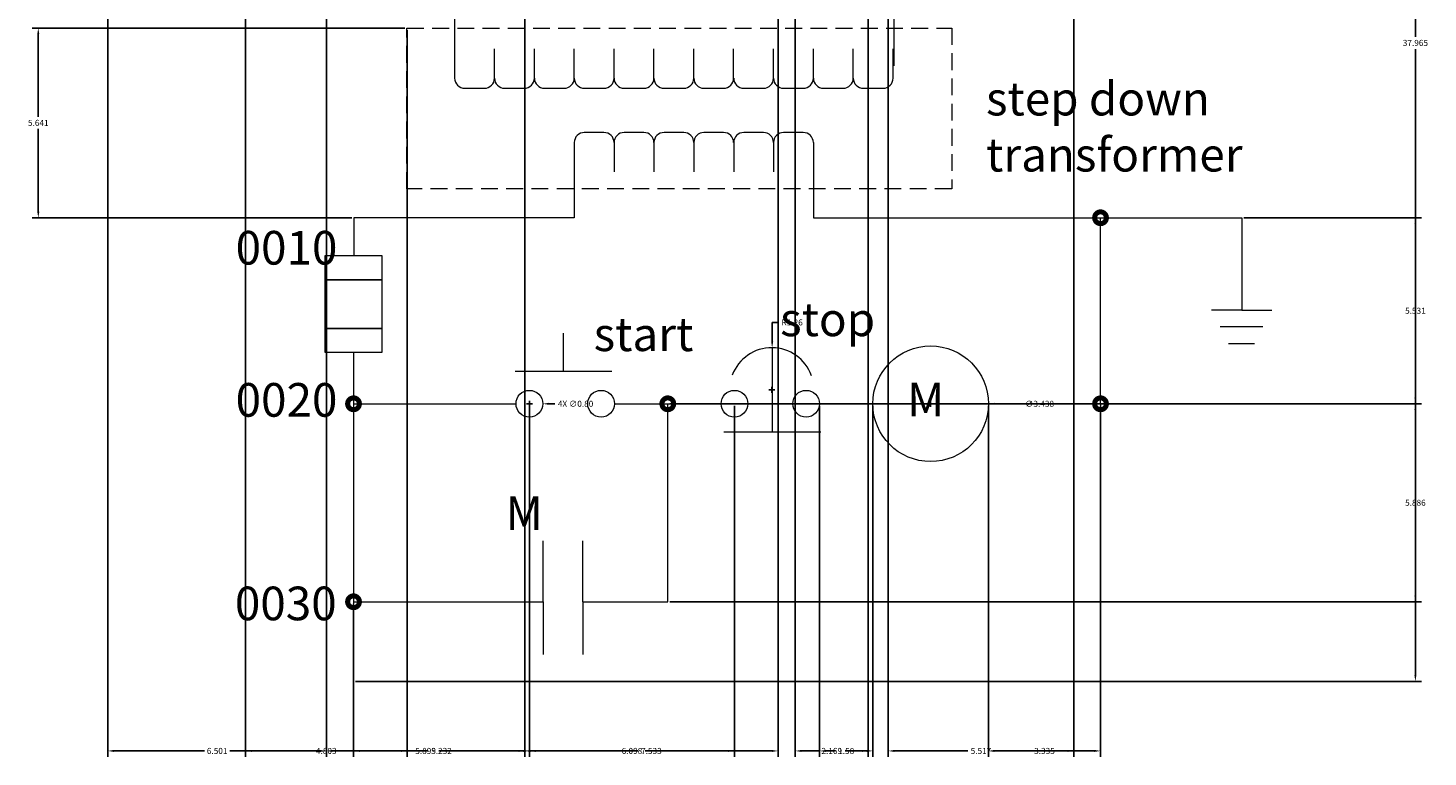
# Model space of a CAD drawing. Units: millimetres. Extents: x 39.4 to 81, y 9.5 to 52.5.
# Tile 1 of 2: x 39.4 to 81, y 9.5 to 31.2. Entities that reach past the tile are written whole.
import ezdxf

# ---------------------------------------------------------------- set-up
doc = ezdxf.new("R2010")
doc.units = ezdxf.units.MM
doc.header["$MEASUREMENT"] = 0
doc.linetypes.add('HIDDENX2', pattern=[0.75, 0.5, -0.25])
for name, color, linetype, lineweight in [('A-ANNO-DIMS', 2, 'Continuous', 18), ('E-ANNO-TEXT', 7, 'Continuous', 13), ('E-CTRL-DEVC', 7, 'Continuous', 18), ('E-CTRL-WIRE', 7, 'Continuous', 13), ('E-DIAG-CONN', 7, 'Continuous', 18), ('E-DIAG-PROT', 7, 'Continuous', 18), ('E-EQPM-BNDY', 8, 'HIDDENX2', 13), ('E-POWR-GRND', 7, 'Continuous', 18), ('E-POWR-WIRE', 7, 'Continuous', 18), ('E-POWR-XFMR', 7, 'Continuous', 18)]:
    doc.layers.add(name, color=color, linetype=linetype, lineweight=lineweight)
doc.styles.get("Standard").update_dxf_attribs({"font": 'arial.ttf'})
doc.dimstyles.get("Standard").update_dxf_attribs({"dimtxt": 0.18, "dimasz": 0.18, "dimexe": 0.18, "dimexo": 0.0625, "dimgap": 0.09, "dimtad": 0, "dimtih": 1, "dimtoh": 1, "dimdec": 4, "dimzin": 0, "dimdsep": 46, "dimtxsty": 'Standard', "dimcen": 0.09, "dimadec": 0, "dimazin": 0, "dimtfac": 1, "dimtdec": 4, "dimtofl": 0, "dimtmove": 0, "dimatfit": 3, "dimfxl": 1, "dimtolj": 1, "dimtzin": 0, "dimarcsym": 0})

# ---------------------------------------------------------------- blocks, each defined once
blk = doc.blocks.new('WIRE-JUNCTION')
at = {"const_width": 0.15}
blk.add_lwpolyline([(0, 0.175, 1), (0.35, 0.175, 1)], format="xyb", close=True, dxfattribs=at)
blk = doc.blocks.new('*D9')
at = {"layer": 'A-ANNO-DIMS', "color": 0, "lineweight": -2, "transparency": 16777216}
for p, q in [((50.604, 31.159), (39.52, 31.159)), ((39.7, 30.979), (39.7, 28.521)), ((39.7, 25.698), (39.7, 28.157)), ((49.021, 25.518), (39.52, 25.518))]:
    blk.add_line(p, q, dxfattribs=at)
at = {"layer": 'A-ANNO-DIMS', "color": 0, "transparency": 16777216}
for points in [[(39.67, 30.979), (39.73, 30.979), (39.7, 31.159)], [(39.67, 25.698), (39.73, 25.698), (39.7, 25.518)]]:
    blk.add_solid(points, dxfattribs=at)
at = {"layer": 'Defpoints', "color": 0, "transparency": 16777216}
for p in [(50.667, 31.159), (39.7, 25.518), (49.084, 25.518)]:
    blk.add_point(p, dxfattribs=at)
at = {"layer": 'A-ANNO-DIMS', "color": 0, "transparency": 16777216, "insert": (39.7, 28.339), "char_height": 0.18, "attachment_point": 5}
blk.add_mtext('\\A1;5.641', dxfattribs=at)
blk = doc.blocks.new('*D10')
at = {"layer": 'A-ANNO-DIMS', "color": 0, "lineweight": -2, "transparency": 16777216}
for p, q in [((75.556, 25.518), (80.841, 25.518)), ((80.661, 25.338), (80.661, 22.935)), ((80.661, 20.167), (80.661, 22.571)), ((71.358, 19.987), (80.841, 19.987))]:
    blk.add_line(p, q, dxfattribs=at)
at = {"layer": 'A-ANNO-DIMS', "color": 0, "transparency": 16777216}
for points in [[(80.631, 25.338), (80.691, 25.338), (80.661, 25.518)], [(80.631, 20.167), (80.691, 20.167), (80.661, 19.987)]]:
    blk.add_solid(points, dxfattribs=at)
at = {"layer": 'Defpoints', "color": 0, "transparency": 16777216}
for p in [(75.494, 25.518), (71.295, 19.987), (80.661, 19.987)]:
    blk.add_point(p, dxfattribs=at)
at = {"layer": 'A-ANNO-DIMS', "color": 0, "transparency": 16777216, "insert": (80.661, 22.753), "char_height": 0.18, "attachment_point": 5}
blk.add_mtext('\\A1;5.531', dxfattribs=at)
blk = doc.blocks.new('*D11')
at = {"layer": 'A-ANNO-DIMS', "color": 0, "lineweight": -2, "transparency": 16777216}
for p, q in [((58.486, 19.987), (80.841, 19.987)), ((80.661, 19.807), (80.661, 17.226)), ((80.661, 14.282), (80.661, 16.863)), ((58.486, 14.102), (80.841, 14.102))]:
    blk.add_line(p, q, dxfattribs=at)
at = {"layer": 'A-ANNO-DIMS', "color": 0, "transparency": 16777216}
for points in [[(80.631, 19.807), (80.691, 19.807), (80.661, 19.987)], [(80.631, 14.282), (80.691, 14.282), (80.661, 14.102)]]:
    blk.add_solid(points, dxfattribs=at)
at = {"layer": 'Defpoints', "color": 0, "transparency": 16777216}
for p in [(58.424, 19.987), (58.424, 14.102), (80.661, 14.102)]:
    blk.add_point(p, dxfattribs=at)
at = {"layer": 'A-ANNO-DIMS', "color": 0, "transparency": 16777216, "insert": (80.661, 17.045), "char_height": 0.18, "attachment_point": 5}
blk.add_mtext('\\A1;5.886', dxfattribs=at)
blk = doc.blocks.new('*D12')
at = {"layer": 'A-ANNO-DIMS', "color": 0, "lineweight": -2, "transparency": 16777216}
for p, q in [((41.769, 37.833), (41.769, 9.486)), ((48.27, 37.833), (48.27, 9.486)), ((41.949, 9.666), (44.643, 9.666)), ((48.09, 9.666), (45.396, 9.666))]:
    blk.add_line(p, q, dxfattribs=at)
at = {"layer": 'A-ANNO-DIMS', "color": 0, "transparency": 16777216}
for points in [[(41.949, 9.696), (41.949, 9.636), (41.769, 9.666)], [(48.09, 9.696), (48.09, 9.636), (48.27, 9.666)]]:
    blk.add_solid(points, dxfattribs=at)
at = {"layer": 'Defpoints', "color": 0, "transparency": 16777216}
for p in [(41.769, 37.896), (48.27, 37.896), (48.27, 9.666)]:
    blk.add_point(p, dxfattribs=at)
at = {"layer": 'A-ANNO-DIMS', "color": 0, "transparency": 16777216, "insert": (45.02, 9.666), "char_height": 0.18, "attachment_point": 5}
blk.add_mtext('\\A1;6.501', dxfattribs=at)
blk = doc.blocks.new('*D13')
at = {"layer": 'A-ANNO-DIMS', "color": 0, "lineweight": -2, "transparency": 16777216}
for p, q in [((48.27, 37.833), (48.27, 9.486)), ((54.169, 37.833), (54.169, 9.486)), ((48.45, 9.666), (50.826, 9.666)), ((53.989, 9.666), (51.614, 9.666))]:
    blk.add_line(p, q, dxfattribs=at)
at = {"layer": 'A-ANNO-DIMS', "color": 0, "transparency": 16777216}
for points in [[(48.45, 9.696), (48.45, 9.636), (48.27, 9.666)], [(53.989, 9.696), (53.989, 9.636), (54.169, 9.666)]]:
    blk.add_solid(points, dxfattribs=at)
at = {"layer": 'Defpoints', "color": 0, "transparency": 16777216}
for p in [(48.27, 37.896), (54.169, 37.896), (54.169, 9.666)]:
    blk.add_point(p, dxfattribs=at)
at = {"layer": 'A-ANNO-DIMS', "color": 0, "transparency": 16777216, "insert": (51.22, 9.666), "char_height": 0.18, "attachment_point": 5}
blk.add_mtext('\\A1;5.899', dxfattribs=at)
blk = doc.blocks.new('*D14')
at = {"layer": 'A-ANNO-DIMS', "color": 0, "lineweight": -2, "transparency": 16777216}
for p, q in [((54.169, 37.833), (54.169, 9.486)), ((61.702, 36.591), (61.702, 9.486)), ((54.349, 9.666), (57.543, 9.666)), ((61.522, 9.666), (58.329, 9.666))]:
    blk.add_line(p, q, dxfattribs=at)
at = {"layer": 'A-ANNO-DIMS', "color": 0, "transparency": 16777216}
for points in [[(54.349, 9.696), (54.349, 9.636), (54.169, 9.666)], [(61.522, 9.696), (61.522, 9.636), (61.702, 9.666)]]:
    blk.add_solid(points, dxfattribs=at)
at = {"layer": 'Defpoints', "color": 0, "transparency": 16777216}
for p in [(54.169, 37.896), (61.702, 36.653), (61.702, 9.666)]:
    blk.add_point(p, dxfattribs=at)
at = {"layer": 'A-ANNO-DIMS', "color": 0, "transparency": 16777216, "insert": (57.936, 9.666), "char_height": 0.18, "attachment_point": 5}
blk.add_mtext('\\A1;7.533', dxfattribs=at)
blk = doc.blocks.new('*D15')
at = {"layer": 'A-ANNO-DIMS', "color": 0, "lineweight": -2, "transparency": 16777216}
for p, q in [((64.384, 37.833), (64.384, 9.486)), ((62.215, 36.591), (62.215, 9.486)), ((62.395, 9.666), (62.904, 9.666)), ((64.204, 9.666), (63.695, 9.666))]:
    blk.add_line(p, q, dxfattribs=at)
at = {"layer": 'A-ANNO-DIMS', "color": 0, "transparency": 16777216}
for points in [[(62.395, 9.696), (62.395, 9.636), (62.215, 9.666)], [(64.204, 9.696), (64.204, 9.636), (64.384, 9.666)]]:
    blk.add_solid(points, dxfattribs=at)
at = {"layer": 'Defpoints', "color": 0, "transparency": 16777216}
for p in [(64.384, 37.896), (62.215, 36.653), (64.384, 9.666)]:
    blk.add_point(p, dxfattribs=at)
at = {"layer": 'A-ANNO-DIMS', "color": 0, "transparency": 16777216, "insert": (63.3, 9.666), "char_height": 0.18, "attachment_point": 5}
blk.add_mtext('\\A1;2.169', dxfattribs=at)
blk = doc.blocks.new('*D16')
at = {"layer": 'A-ANNO-DIMS', "color": 0, "lineweight": -2, "transparency": 16777216}
for p, q in [((64.98, 37.879), (64.98, 9.486)), ((70.498, 37.833), (70.498, 9.486)), ((65.16, 9.666), (67.345, 9.666)), ((70.318, 9.666), (68.133, 9.666))]:
    blk.add_line(p, q, dxfattribs=at)
at = {"layer": 'A-ANNO-DIMS', "color": 0, "transparency": 16777216}
for points in [[(65.16, 9.696), (65.16, 9.636), (64.98, 9.666)], [(70.318, 9.696), (70.318, 9.636), (70.498, 9.666)]]:
    blk.add_solid(points, dxfattribs=at)
at = {"layer": 'Defpoints', "color": 0, "transparency": 16777216}
for p in [(64.98, 37.941), (70.498, 37.896), (70.498, 9.666)]:
    blk.add_point(p, dxfattribs=at)
at = {"layer": 'A-ANNO-DIMS', "color": 0, "transparency": 16777216, "insert": (67.739, 9.666), "char_height": 0.18, "attachment_point": 5}
blk.add_mtext('\\A1;5.517', dxfattribs=at)
blk = doc.blocks.new('*D17')
at = {"layer": 'A-ANNO-DIMS', "color": 0, "lineweight": -2, "transparency": 16777216}
for p, q in [((54.309, 19.925), (54.309, 9.486)), ((49.077, 14.039), (49.077, 9.486)), ((49.257, 9.666), (51.3, 9.666)), ((54.129, 9.666), (52.085, 9.666))]:
    blk.add_line(p, q, dxfattribs=at)
at = {"layer": 'A-ANNO-DIMS', "color": 0, "transparency": 16777216}
for points in [[(49.257, 9.696), (49.257, 9.636), (49.077, 9.666)], [(54.129, 9.696), (54.129, 9.636), (54.309, 9.666)]]:
    blk.add_solid(points, dxfattribs=at)
at = {"layer": 'Defpoints', "color": 0, "transparency": 16777216}
for p in [(54.309, 19.987), (49.077, 14.102), (54.309, 9.666)]:
    blk.add_point(p, dxfattribs=at)
at = {"layer": 'A-ANNO-DIMS', "color": 0, "transparency": 16777216, "insert": (51.693, 9.666), "char_height": 0.18, "attachment_point": 5}
blk.add_mtext('\\A1;5.232', dxfattribs=at)
blk = doc.blocks.new('*D18')
at = {"layer": 'A-ANNO-DIMS', "color": 0, "lineweight": -2, "transparency": 16777216}
for p, q in [((54.309, 19.925), (54.309, 9.486)), ((60.407, 19.925), (60.407, 9.486)), ((54.489, 9.666), (56.964, 9.666)), ((60.227, 9.666), (57.752, 9.666))]:
    blk.add_line(p, q, dxfattribs=at)
at = {"layer": 'A-ANNO-DIMS', "color": 0, "transparency": 16777216}
for points in [[(54.489, 9.696), (54.489, 9.636), (54.309, 9.666)], [(60.227, 9.696), (60.227, 9.636), (60.407, 9.666)]]:
    blk.add_solid(points, dxfattribs=at)
at = {"layer": 'Defpoints', "color": 0, "transparency": 16777216}
for p in [(54.309, 19.987), (60.407, 19.987), (60.407, 9.666)]:
    blk.add_point(p, dxfattribs=at)
at = {"layer": 'A-ANNO-DIMS', "color": 0, "transparency": 16777216, "insert": (57.358, 9.666), "char_height": 0.18, "attachment_point": 5}
blk.add_mtext('\\A1;6.098', dxfattribs=at)
blk = doc.blocks.new('*D19')
at = {"layer": 'A-ANNO-DIMS', "color": 0, "lineweight": -2, "transparency": 16777216}
for p, q in [((62.938, 19.925), (62.938, 9.486)), ((64.522, 19.925), (64.522, 9.486)), ((63.118, 9.666), (63.414, 9.666)), ((64.342, 9.666), (64.045, 9.666))]:
    blk.add_line(p, q, dxfattribs=at)
at = {"layer": 'A-ANNO-DIMS', "color": 0, "transparency": 16777216}
for points in [[(63.118, 9.696), (63.118, 9.636), (62.938, 9.666)], [(64.342, 9.696), (64.342, 9.636), (64.522, 9.666)]]:
    blk.add_solid(points, dxfattribs=at)
at = {"layer": 'Defpoints', "color": 0, "transparency": 16777216}
for p in [(62.938, 19.987), (64.522, 19.987), (64.522, 9.666)]:
    blk.add_point(p, dxfattribs=at)
at = {"layer": 'A-ANNO-DIMS', "color": 0, "transparency": 16777216, "insert": (63.73, 9.666), "char_height": 0.18, "attachment_point": 5}
blk.add_mtext('\\A1;1.58', dxfattribs=at)
blk = doc.blocks.new('*D20')
at = {"layer": 'A-ANNO-DIMS', "color": 0, "lineweight": -2, "transparency": 16777216}
for p, q in [((67.96, 19.925), (67.96, 9.486)), ((71.295, 19.925), (71.295, 9.486)), ((68.14, 9.666), (69.233, 9.666)), ((71.115, 9.666), (70.022, 9.666))]:
    blk.add_line(p, q, dxfattribs=at)
at = {"layer": 'A-ANNO-DIMS', "color": 0, "transparency": 16777216}
for points in [[(68.14, 9.696), (68.14, 9.636), (67.96, 9.666)], [(71.115, 9.696), (71.115, 9.636), (71.295, 9.666)]]:
    blk.add_solid(points, dxfattribs=at)
at = {"layer": 'Defpoints', "color": 0, "transparency": 16777216}
for p in [(67.96, 19.987), (71.295, 19.987), (71.295, 9.666)]:
    blk.add_point(p, dxfattribs=at)
at = {"layer": 'A-ANNO-DIMS', "color": 0, "transparency": 16777216, "insert": (69.628, 9.666), "char_height": 0.18, "attachment_point": 5}
blk.add_mtext('\\A1;3.335', dxfattribs=at)
blk = doc.blocks.new('*D22')
at = {"layer": 'A-ANNO-DIMS', "color": 0, "lineweight": -2, "transparency": 16777216}
for p, q in [((67.825, 49.7), (80.841, 49.7)), ((80.661, 49.52), (80.661, 30.899)), ((80.661, 11.915), (80.661, 30.535)), ((49.139, 11.735), (80.841, 11.735))]:
    blk.add_line(p, q, dxfattribs=at)
at = {"layer": 'A-ANNO-DIMS', "color": 0, "transparency": 16777216}
for points in [[(80.631, 49.52), (80.691, 49.52), (80.661, 49.7)], [(80.631, 11.915), (80.691, 11.915), (80.661, 11.735)]]:
    blk.add_solid(points, dxfattribs=at)
at = {"layer": 'Defpoints', "color": 0, "transparency": 16777216}
for p in [(67.763, 49.7), (49.077, 11.735), (80.661, 11.735)]:
    blk.add_point(p, dxfattribs=at)
at = {"layer": 'A-ANNO-DIMS', "color": 0, "transparency": 16777216, "insert": (80.661, 30.717), "char_height": 0.18, "attachment_point": 5}
blk.add_mtext('\\A1;37.965', dxfattribs=at)
blk = doc.blocks.new('*D23')
at = {"layer": 'A-ANNO-DIMS', "color": 0, "lineweight": -2, "transparency": 16777216}
for p, q in [((45.864, 34.781), (45.864, 9.486)), ((50.667, 31.097), (50.667, 9.486)), ((46.044, 9.666), (47.868, 9.666)), ((50.487, 9.666), (48.663, 9.666))]:
    blk.add_line(p, q, dxfattribs=at)
at = {"layer": 'A-ANNO-DIMS', "color": 0, "transparency": 16777216}
for points in [[(46.044, 9.696), (46.044, 9.636), (45.864, 9.666)], [(50.487, 9.696), (50.487, 9.636), (50.667, 9.666)]]:
    blk.add_solid(points, dxfattribs=at)
at = {"layer": 'Defpoints', "color": 0, "transparency": 16777216}
for p in [(45.864, 34.843), (50.667, 31.159), (50.667, 9.666)]:
    blk.add_point(p, dxfattribs=at)
at = {"layer": 'A-ANNO-DIMS', "color": 0, "transparency": 16777216, "insert": (48.265, 9.666), "char_height": 0.18, "attachment_point": 5}
blk.add_mtext('\\A1;4.803', dxfattribs=at)
blk = doc.blocks.new('*D25')
at = {"layer": 'A-ANNO-DIMS', "color": 0, "lineweight": -2, "transparency": 16777216}
for p, q in [((66.241, 19.897), (66.241, 20.077)), ((66.151, 19.987), (66.331, 19.987)), ((68.992, 19.987), (68.14, 19.987))]:
    blk.add_line(p, q, dxfattribs=at)
at = {"layer": 'A-ANNO-DIMS', "color": 0, "transparency": 16777216}
blk.add_solid([(68.14, 20.017), (68.14, 19.957), (67.96, 19.987)], dxfattribs=at)
at = {"layer": 'Defpoints', "color": 0, "transparency": 16777216}
for p in [(64.522, 19.988), (67.96, 19.987)]:
    blk.add_point(p, dxfattribs=at)
at = {"layer": 'A-ANNO-DIMS', "color": 0, "transparency": 16777216, "insert": (69.483, 19.987), "char_height": 0.18, "attachment_point": 5}
blk.add_mtext('\\A1;∅3.438', dxfattribs=at)
blk = doc.blocks.new('*D27')
at = {"layer": 'A-ANNO-DIMS', "color": 0, "lineweight": -2, "transparency": 16777216}
for p, q in [((61.533, 22.407), (61.529, 21.834)), ((61.713, 22.407), (61.533, 22.407)), ((61.516, 20.308), (61.516, 20.488)), ((61.426, 20.398), (61.606, 20.398))]:
    blk.add_line(p, q, dxfattribs=at)
at = {"layer": 'A-ANNO-DIMS', "color": 0, "transparency": 16777216}
blk.add_solid([(61.499, 21.834), (61.559, 21.833), (61.527, 21.654)], dxfattribs=at)
at = {"layer": 'Defpoints', "color": 0, "transparency": 16777216}
for p in [(61.527, 21.654), (61.516, 20.398)]:
    blk.add_point(p, dxfattribs=at)
at = {"layer": 'A-ANNO-DIMS', "color": 0, "transparency": 16777216, "insert": (62.123, 22.407), "char_height": 0.18, "attachment_point": 5}
blk.add_mtext('\\A1;R1.26', dxfattribs=at)
blk = doc.blocks.new('*D30')
at = {"layer": 'A-ANNO-DIMS', "color": 0, "lineweight": -2, "transparency": 16777216}
for p, q in [((54.309, 19.897), (54.309, 20.077)), ((54.219, 19.987), (54.399, 19.987)), ((55.067, 19.987), (54.887, 19.987))]:
    blk.add_line(p, q, dxfattribs=at)
at = {"layer": 'A-ANNO-DIMS', "color": 0, "transparency": 16777216}
blk.add_solid([(54.887, 20.017), (54.887, 19.957), (54.707, 19.987)], dxfattribs=at)
at = {"layer": 'Defpoints', "color": 0, "transparency": 16777216}
for p in [(53.91, 19.988), (54.707, 19.987)]:
    blk.add_point(p, dxfattribs=at)
at = {"layer": 'A-ANNO-DIMS', "color": 0, "transparency": 16777216, "insert": (55.681, 19.987), "char_height": 0.18, "attachment_point": 5}
blk.add_mtext('\\A1;4X ∅0.80', dxfattribs=at)

msp = doc.modelspace()

# ---------------------------------------------------------------- linework, layer by layer
at = {"layer": 'E-CTRL-DEVC'}
for p, q in [((55.3214, 20.9583), (55.3214, 22.0866)), ((61.5374, 19.1486), (61.5374, 21.6536)), ((53.8794, 20.9583), (56.7635, 20.9583)), ((60.0954, 19.1486), (62.9795, 19.1486)), ((54.7206, 14.1015), (54.7206, 15.9122)), ((55.8983, 14.1015), (55.8983, 15.9122)), ((54.7206, 14.1015), (54.7206, 12.5378)), ((55.8983, 14.1015), (55.8983, 12.5378))]:
    msp.add_line(p, q, dxfattribs=at)
for centre, radius in [((66.2412, 19.9875), 1.719), ((54.3088, 19.9875), 0.3986), ((56.4408, 19.9875), 0.3986), ((60.4071, 19.9875), 0.3986), ((62.5391, 19.9875), 0.3986)]:
    msp.add_circle(centre, radius, dxfattribs=at)
msp.add_arc((61.5163, 20.3975), 1.2563, 19.8001, 159.24973, dxfattribs=at)
at = {"layer": 'E-CTRL-WIRE'}
for p, q in [((55.6412, 26.8815), (55.6412, 25.5184)), ((62.7546, 26.8815), (62.7546, 25.5184)), ((55.6412, 25.5184), (49.0837, 25.5184)), ((49.0837, 25.5184), (49.0837, 24.3951)), ((62.7546, 25.5184), (75.4939, 25.5184)), ((71.2952, 19.9875), (71.2952, 25.5184)), ((75.4939, 25.5184), (75.4939, 22.7727)), ((49.0765, 21.5084), (49.0765, 11.7347)), ((49.0765, 19.9875), (53.9102, 19.9875)), ((56.8394, 19.9875), (60.0085, 19.9875)), ((58.424, 14.1015), (58.424, 19.9875)), ((62.9377, 19.9875), (64.5222, 19.9875)), ((67.9602, 19.9875), (71.2952, 19.9875)), ((71.2952, 19.9875), (71.2952, 16.0213)), ((49.0765, 14.1015), (54.7206, 14.1015)), ((55.8983, 14.1015), (58.424, 14.1015))]:
    msp.add_line(p, q, dxfattribs=at)
at = {"layer": 'E-DIAG-PROT'}
for p, q in [((48.2375, 24.3951), (49.9155, 24.3951)), ((48.2375, 23.6734), (48.2375, 24.3951)), ((49.9155, 24.3951), (49.9155, 23.6734)), ((49.9155, 23.6734), (48.2375, 23.6734)), ((48.2375, 23.6734), (49.9155, 23.6734)), ((48.2375, 22.9518), (48.2375, 23.6734)), ((49.9155, 23.6734), (49.9155, 22.9518)), ((48.2375, 22.2301), (48.2375, 22.9518)), ((49.9155, 22.9518), (49.9155, 22.2301)), ((49.9155, 22.2301), (48.2375, 22.2301))]:
    msp.add_line(p, q, dxfattribs=at)
msp.add_lwpolyline([(49.9155, 22.2301), (49.9155, 21.5084), (48.2375, 21.5084), (48.2375, 22.2301)], close=True, dxfattribs=at)
at = {"layer": 'E-EQPM-BNDY'}
msp.add_lwpolyline([(50.6667, 31.1595), (66.8695, 31.1595), (66.8695, 26.3781), (50.6667, 26.3781)], close=True, dxfattribs=at)
at = {"layer": 'E-POWR-GRND'}
for p, q in [((75.4939, 22.7727), (74.5999, 22.7727)), ((75.4939, 22.7727), (76.388, 22.7727)), ((76.126, 22.2727), (74.8505, 22.2727)), ((75.8754, 21.7727), (75.1011, 21.7727))]:
    msp.add_line(p, q, dxfattribs=at)
at = {"layer": 'E-POWR-WIRE'}
for p, q in [((52.0845, 32.2872), (52.0845, 30.0317)), ((65.1455, 32.2872), (65.1455, 30.0317))]:
    msp.add_line(p, q, dxfattribs=at)
at = {"layer": 'E-POWR-XFMR'}
for p, q in [((65.1248, 29.6678), (65.1248, 30.54)), ((52.0845, 30.0317), (52.0845, 29.6678)), ((62.7546, 27.7537), (62.7546, 26.8815))]:
    msp.add_line(p, q, dxfattribs=at)
for points in [[(52.3845, 29.3678), (52.9691, 29.3678, 0.4142136), (53.2691, 29.6678), (53.2691, 30.54)], [(53.27, 29.6678, 0.4142136), (53.57, 29.3678), (54.1546, 29.3678, 0.4142136), (54.4546, 29.6678), (54.4546, 30.54)], [(54.4556, 29.6678, 0.4142136), (54.7556, 29.3678), (55.3402, 29.3678, 0.4142136), (55.6402, 29.6678), (55.6402, 30.54)], [(55.6412, 29.6678, 0.4142136), (55.9412, 29.3678), (56.5258, 29.3678, 0.4142136), (56.8258, 29.6678), (56.8258, 30.54)], [(56.8267, 29.6678, 0.4142136), (57.1267, 29.3678), (57.7113, 29.3678, 0.4142136), (58.0113, 29.6678), (58.0113, 30.54)], [(58.0123, 29.6678, 0.4142136), (58.3123, 29.3678), (58.8969, 29.3678, 0.4142136), (59.1969, 29.6678), (59.1969, 30.54)], [(59.1979, 29.6678, 0.4142136), (59.4979, 29.3678), (60.0825, 29.3678, 0.4142136), (60.3825, 29.6678), (60.3825, 30.54)], [(60.3834, 29.6678, 0.4142136), (60.6834, 29.3678), (61.268, 29.3678, 0.4142136), (61.568, 29.6678), (61.568, 30.54)], [(61.569, 29.6678, 0.4142136), (61.869, 29.3678), (62.4536, 29.3678, 0.4142136), (62.7536, 29.6678), (62.7536, 30.54)], [(62.7546, 29.6678, 0.4142136), (63.0546, 29.3678), (63.6392, 29.3678, 0.4142136), (63.9392, 29.6678), (63.9392, 30.54)], [(63.9401, 29.6678, 0.4142136), (64.2401, 29.3678), (64.8248, 29.3678)], [(56.8258, 27.7537, 0.4142136), (56.5258, 28.0537), (55.9412, 28.0537, 0.4142136), (55.6412, 27.7537), (55.6412, 26.8815)], [(58.0113, 27.7537, 0.4142136), (57.7113, 28.0537), (57.1267, 28.0537, 0.4142136), (56.8267, 27.7537), (56.8267, 26.8815)], [(59.1969, 27.7537, 0.4142136), (58.8969, 28.0537), (58.3123, 28.0537, 0.4142136), (58.0123, 27.7537), (58.0123, 26.8815)], [(60.3825, 27.7537, 0.4142136), (60.0825, 28.0537), (59.4979, 28.0537, 0.4142136), (59.1979, 27.7537), (59.1979, 26.8815)], [(61.568, 27.7537, 0.4142136), (61.268, 28.0537), (60.6834, 28.0537, 0.4142136), (60.3834, 27.7537), (60.3834, 26.8815)], [(62.7536, 27.7537, 0.4142136), (62.4536, 28.0537), (61.869, 28.0537, 0.4142136), (61.569, 27.7537), (61.569, 26.8815)]]:
    msp.add_lwpolyline(points, format="xyb", dxfattribs=at)
for centre, start, end in [((52.3845, 29.6678), 180, 270), ((64.8248, 29.6678), 270, 0)]:
    msp.add_arc(centre, 0.3, start, end, dxfattribs=at)

# ---------------------------------------------------------------- block references
at = {"layer": 'E-DIAG-CONN'}
for p in [(71.12, 25.343), (48.9013, 19.812), (58.2488, 19.812), (71.12, 19.812), (48.9013, 13.9261)]:
    msp.add_blockref('WIRE-JUNCTION', p, dxfattribs=at)

# ---------------------------------------------------------------- texts
at = {"layer": 'E-ANNO-TEXT', "char_height": 1, "attachment_point": 1}
for s, width, insert in [('step down transformer', 14.406916, (67.8892, 29.5599)), ('0010', 2.308794, (45.5688, 25.126)), ('stop', 2.308794, (61.7655, 22.9978)), ('start', 2.308794, (56.2187, 22.5544)), ('0020', 2.308794, (45.5688, 20.6035)), ('M', 2.308794, (65.5414, 20.6168)), ('M', 2.308794, (53.6006, 17.2338)), ('0030', 2.308794, (45.5468, 14.5513))]:
    msp.add_mtext_dynamic_manual_height_columns(s, width=width, gutter_width=1, heights=[0], dxfattribs=dict(at, insert=insert))

# ---------------------------------------------------------------- dimensions: what is measured, and where the dimension line sits
at = {"layer": 'A-ANNO-DIMS'}
for base, p1, p2, picture, middle in [((80.6609, 11.7347), (67.763, 49.6995), (49.0765, 11.7347), '*D22', (80.6609, 30.7171)), ((39.7004, 25.5184), (50.6667, 31.1595), (49.0837, 25.5184), '*D9', (39.7004, 28.339)), ((80.6609, 19.9875), (75.4939, 25.5184), (71.2952, 19.9875), '*D10', (80.6609, 22.753)), ((80.6609, 14.1015), (58.424, 19.9875), (58.424, 14.1015), '*D11', (80.6609, 17.0445))]:
    dim = msp.add_linear_dim(base=base, p1=p1, p2=p2, angle=90, dimstyle='Standard', override={"dimdec": 3, "dimlfac": 1, "dimrnd": 0, "dimzin": 0, "dimdsep": 46, "dimlunit": 2}, dxfattribs=at)
    dim.commit()
    dim.dimension.update_dxf_attribs({"geometry": picture, "text_midpoint": middle})
for base, p1, p2, override, picture, middle in [((48.2702, 9.6662), (41.7689, 37.8959), (48.2702, 37.8959), {"dimdec": 3, "dimlfac": 1, "dimrnd": 0, "dimzin": 0, "dimdsep": 46, "dimlunit": 2}, '*D12', (45.0195, 9.6662)), ((54.1694, 9.6662), (48.2702, 37.8959), (54.1694, 37.8959), {"dimdec": 3, "dimlfac": 1, "dimrnd": 0, "dimzin": 0, "dimdsep": 46, "dimlunit": 2}, '*D13', (51.2198, 9.6662)), ((61.7024, 9.6662), (54.1694, 37.8959), (61.7024, 36.6533), {"dimdec": 3, "dimlfac": 1, "dimrnd": 0, "dimzin": 0, "dimdsep": 46, "dimlunit": 2}, '*D14', (57.9359, 9.6662)), ((64.3842, 9.6662), (62.2151, 36.6533), (64.3842, 37.8959), {"dimdec": 3, "dimlfac": 1, "dimrnd": 0, "dimzin": 0, "dimdsep": 46, "dimlunit": 2}, '*D15', (63.2997, 9.6662)), ((70.4975, 9.6662), (64.9801, 37.9414), (70.4975, 37.8959), {"dimdec": 3, "dimlfac": 1, "dimrnd": 0, "dimzin": 0, "dimdsep": 46, "dimlunit": 2}, '*D16', (67.7388, 9.6662)), ((50.6667, 9.6662), (45.8641, 34.8433), (50.6667, 31.1595), {"dimdec": 3, "dimlfac": 1, "dimrnd": 0, "dimzin": 0, "dimdsep": 46, "dimlunit": 2}, '*D23', (48.2654, 9.6662)), ((54.3088, 9.6662), (49.0765, 14.1015), (54.3088, 19.9875), {"dimdec": 3, "dimlfac": 1, "dimrnd": 0, "dimzin": 0, "dimdsep": 46, "dimlunit": 2}, '*D17', (51.6927, 9.6662)), ((60.4071, 9.6662), (54.3088, 19.9875), (60.4071, 19.9875), {"dimdec": 3, "dimlfac": 1, "dimrnd": 0, "dimzin": 0, "dimdsep": 46, "dimlunit": 2}, '*D18', (57.358, 9.6662)), ((64.5222, 9.6662), (62.9377, 19.9875), (64.5222, 19.9875), {"dimdec": 2, "dimlfac": 1, "dimrnd": 0, "dimzin": 0, "dimdsep": 46, "dimlunit": 2}, '*D19', (63.73, 9.6662)), ((71.2952, 9.6662), (67.9602, 19.9875), (71.2952, 19.9875), {"dimdec": 3, "dimlfac": 1, "dimrnd": 0, "dimzin": 0, "dimdsep": 46, "dimlunit": 2}, '*D20', (69.6277, 9.6662))]:
    dim = msp.add_linear_dim(base=base, p1=p1, p2=p2, dimstyle='Standard', override=override, dxfattribs=at)
    dim.commit()
    dim.dimension.update_dxf_attribs({"geometry": picture, "text_midpoint": middle})
dim = msp.add_radius_dim(center=(61.5163, 20.3975), mpoint=(61.527, 21.6538), dimstyle='Standard', override={"dimdec": 2, "dimlfac": 1, "dimrnd": 0, "dimzin": 0, "dimdsep": 46, "dimlunit": 2}, dxfattribs=at)
dim.commit()
dim.dimension.update_dxf_attribs({"geometry": '*D27', "text_midpoint": (62.1232, 22.4075), "dimtype": 164})
dim = msp.add_diameter_dim_2p(p1=(53.9102, 19.988), p2=(54.7074, 19.987), text='4X <>', dimstyle='Standard', override={"dimdec": 2, "dimlfac": 1, "dimrnd": 0, "dimzin": 0, "dimdsep": 46, "dimlunit": 2}, dxfattribs=at)
dim.commit()
dim.dimension.update_dxf_attribs({"geometry": '*D30', "text_midpoint": (55.0674, 19.9866)})
dim = msp.add_diameter_dim_2p(p1=(64.5222, 19.988), p2=(67.9602, 19.987), dimstyle='Standard', override={"dimdec": 3, "dimlfac": 1, "dimrnd": 0, "dimzin": 0, "dimdsep": 46, "dimlunit": 2}, dxfattribs=at)
dim.commit()
dim.dimension.update_dxf_attribs({"geometry": '*D25', "text_midpoint": (68.9916, 19.9867), "dimtype": 163})

doc.saveas('drawing.dxf')
